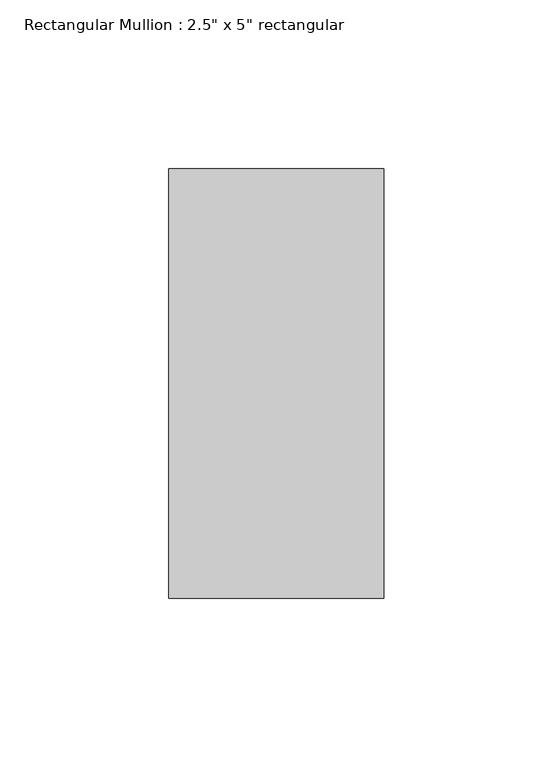
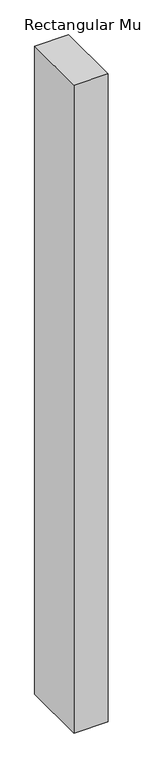
"""IFC4 building model written with IfcOpenShell, lengths in millimetres: member geometry."""

from ifc_helpers import new_model, si_unit, frame, origin, place, context, project, spatial, polyline, outline, extrude, source, transform, mapped, element, save


def member_58fbc06e(model_context):
    return source(origin(), model_context, "Body", "SweptSolid", [
        extrude(outline(polyline([(31.75, 63.5), (31.75, -63.5), (-31.75, -63.5), (-31.75, 63.5), (31.75, 63.5)])), frame((0.0, 0.0, -1276.35), z_axis=(0.0, 0.0, 1.0), x_axis=(1.0, 0.0, 0.0)), (0.0, 0.0, 1.0), 1276.35),
    ])


if __name__ == "__main__":
    model = new_model("IFC4")
    model_context = context("Model", 3, world=origin())
    ifc_project = project(units=[si_unit("LENGTHUNIT", "METRE", prefix="MILLI")], contexts=[model_context])
    site = spatial("IfcSite", under=ifc_project)
    building = spatial("IfcBuilding", under=site)
    placement = place(None, origin())
    member_shape = member_58fbc06e(model_context)
    element("IfcMember", 1, ObjectType="Rectangular Mullion : 2.5\" x 5\" rectangular", at=placement, inside=building, context=model_context, shape_type="MappedRepresentation", body=[
        mapped(member_shape, transform((0.0, 0.0, 0.0), x_axis=(1.0, 0.0, 0.0), y_axis=(0.0, 1.0, 0.0), z_axis=(0.0, 0.0, 1.0))),
    ])
    save(model, "model.ifc")

# Revit data of these elements
# Type "Rectangular Mullion : 2.5\" x 5\" rectangular"
#   built-in parameter 1007304 = 0.416667 (stored number, unit not read)
#   built-in parameter 1007301 = 0.104167 (stored number, unit not read)
#   built-in parameter 1007300 = 0.104167 (stored number, unit not read)
# Element 1 (IfcMember, "Rectangular Mullion : 2.5\" x 5\" rectangular")
#   Materials on its faces: "Aluminum"
# Materials
#   "Aluminum": class "Metal", colour RGB 247 247 247, transparency 0, Description = "Aluminum 6061", Cost = 0
